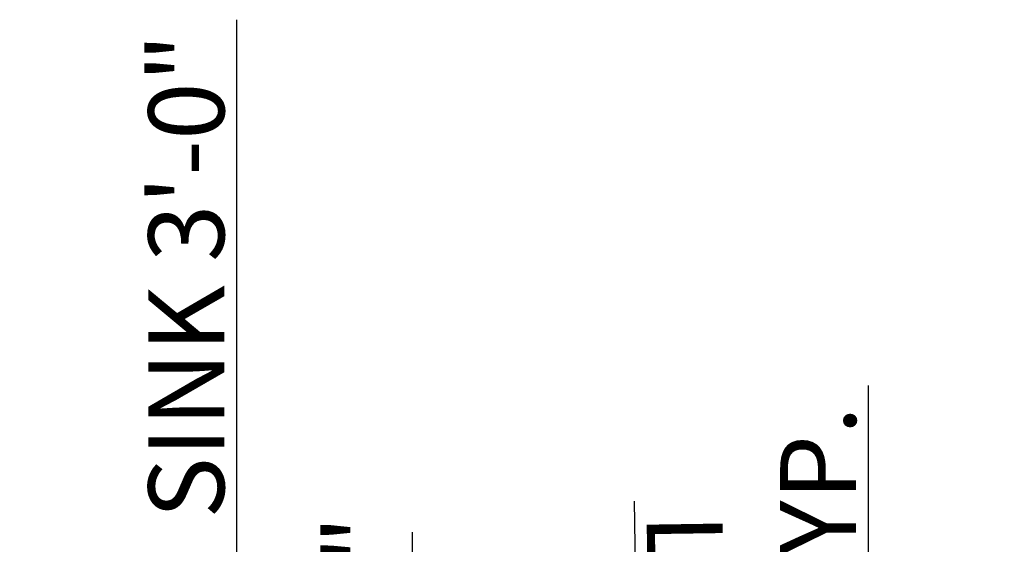
# Model space of a CAD drawing. Units: inches. Extents: x 2901 to 21549, y 2042 to 3828.
# Tile 9 of 10: x 3237 to 3704, y 3579 to 3828. Entities that reach past the tile are written whole.
import ezdxf

# ---------------------------------------------------------------- set-up
doc = ezdxf.new("R2010")
doc.units = ezdxf.units.IN
doc.layers.get('Defpoints').update_dxf_attribs({"color": 1})
doc.layers.add('A-ANNO-DIMS', color=2, linetype='Continuous', lineweight=18)
doc.styles.get("Standard").update_dxf_attribs({"font": 'arial.ttf'})
doc.dimstyles.new('ISO-25', dxfattribs={"dimtxt": 36, "dimasz": 5, "dimexe": 1.25, "dimexo": 0.625, "dimtad": 1, "dimdec": 0, "dimlunit": 3, "dimtxsty": 'Standard', "dimcen": 2.5, "dimadec": 0, "dimazin": 0, "dimtfac": 1, "dimtdec": 0, "dimtmove": 0, "dimatfit": 3, "dimfxl": 1, "dimarcsym": 0})

# ---------------------------------------------------------------- blocks, each defined once
blk = doc.blocks.new('*D36')
at = {"layer": 'A-ANNO-DIMS', "color": 0, "lineweight": -2, "transparency": 16777216}
for p, q in [((3639.47, 3192.64), (3639.47, 3654.44)), ((3634.69, 3192.64), (3640.72, 3192.64)), ((3639.47, 3161.64), (3639.47, 3187.64)), ((3634.69, 3156.64), (3640.72, 3156.64))]:
    blk.add_line(p, q, dxfattribs=at)
at = {"layer": 'A-ANNO-DIMS', "color": 0, "transparency": 16777216}
for points in [[(3638.64, 3187.64), (3640.3, 3187.64), (3639.47, 3192.64)], [(3638.64, 3161.64), (3640.3, 3161.64), (3639.47, 3156.64)]]:
    blk.add_solid(points, dxfattribs=at)
at = {"layer": 'Defpoints', "color": 0, "transparency": 16777216}
for p in [(3634.07, 3192.64), (3639.47, 3192.64), (3634.07, 3156.64)]:
    blk.add_point(p, dxfattribs=at)
at = {"layer": 'A-ANNO-DIMS', "color": 0, "transparency": 16777216, "insert": (3620.21, 3426.04), "char_height": 36, "attachment_point": 5, "rotation": 90}
blk.add_mtext('WINDOW 3\'-0" TYP.', dxfattribs=at)
blk = doc.blocks.new('*D42')
at = {"layer": 'A-ANNO-DIMS', "color": 0, "lineweight": -2, "transparency": 16777216}
for p, q in [((3533.42, 3266.44), (3528.38, 3599.53)), ((3535.49, 3266.47), (3532.17, 3266.42)), ((3533.62, 3253.49), (3533.5, 3261.44)), ((3535.76, 3248.52), (3532.44, 3248.47))]:
    blk.add_line(p, q, dxfattribs=at)
at = {"layer": 'A-ANNO-DIMS', "color": 0, "transparency": 16777216}
for points in [[(3534.33, 3261.45), (3532.66, 3261.43), (3533.42, 3266.44)], [(3534.45, 3253.5), (3532.78, 3253.48), (3533.69, 3248.49)]]:
    blk.add_solid(points, dxfattribs=at)
at = {"layer": 'Defpoints', "color": 0, "transparency": 16777216}
for p in [(3533.42, 3266.44), (3536.11, 3266.48), (3536.39, 3248.53)]:
    blk.add_point(p, dxfattribs=at)
at = {"layer": 'A-ANNO-DIMS', "color": 0, "transparency": 16777216, "insert": (3549.86, 3435.77), "char_height": 36, "attachment_point": 5, "rotation": 270.8679}
blk.add_mtext('LAV 1\'-6" TYP.', dxfattribs=at)
blk = doc.blocks.new('*D59')
at = {"layer": 'A-ANNO-DIMS', "color": 0, "lineweight": -2, "transparency": 16777216}
for p, q in [((3423.1, 3402.33), (3423.1, 3584.77)), ((3420.71, 3402.33), (3424.35, 3402.33)), ((3423.1, 3389.91), (3423.1, 3397.33)), ((3420.71, 3384.91), (3424.35, 3384.91))]:
    blk.add_line(p, q, dxfattribs=at)
at = {"layer": 'A-ANNO-DIMS', "color": 0, "transparency": 16777216}
for points in [[(3422.26, 3397.33), (3423.93, 3397.33), (3423.1, 3402.33)], [(3422.26, 3389.91), (3423.93, 3389.91), (3423.1, 3384.91)]]:
    blk.add_solid(points, dxfattribs=at)
at = {"layer": 'Defpoints', "color": 0, "transparency": 16777216}
for p in [(3420.08, 3402.33), (3423.1, 3402.33), (3420.08, 3384.91)]:
    blk.add_point(p, dxfattribs=at)
at = {"layer": 'A-ANNO-DIMS', "color": 0, "transparency": 16777216, "insert": (3403.86, 3496.05), "char_height": 36, "attachment_point": 5, "rotation": 90}
blk.add_mtext('1\'-5 1/2"', dxfattribs=at)
blk = doc.blocks.new('*D60')
at = {"layer": 'A-ANNO-DIMS', "color": 0, "lineweight": -2, "transparency": 16777216}
for p, q in [((3339.61, 3361.55), (3339.61, 3827.97)), ((3344.38, 3361.55), (3338.36, 3361.55)), ((3339.61, 3330.55), (3339.61, 3356.55)), ((3344.38, 3325.55), (3338.36, 3325.55))]:
    blk.add_line(p, q, dxfattribs=at)
at = {"layer": 'A-ANNO-DIMS', "color": 0, "transparency": 16777216}
for points in [[(3338.78, 3356.55), (3340.44, 3356.55), (3339.61, 3361.55)], [(3338.78, 3330.55), (3340.44, 3330.55), (3339.61, 3325.55)]]:
    blk.add_solid(points, dxfattribs=at)
at = {"layer": 'Defpoints', "color": 0, "transparency": 16777216}
for p in [(3339.61, 3361.55), (3345.01, 3361.55), (3345.01, 3325.55)]:
    blk.add_point(p, dxfattribs=at)
at = {"layer": 'A-ANNO-DIMS', "color": 0, "transparency": 16777216, "insert": (3320.36, 3597.26), "char_height": 36, "attachment_point": 5, "rotation": 90}
blk.add_mtext('KITCHEN SINK 3\'-0"', dxfattribs=at)

msp = doc.modelspace()

# ---------------------------------------------------------------- dimensions: what is measured, and where the dimension line sits
at = {"layer": 'A-ANNO-DIMS'}
for base, p1, p2, angle, text, picture, middle in [((3339.61, 3361.55), (3345.01, 3325.55), (3345.01, 3361.55), 90, 'KITCHEN SINK <>', '*D60', (3320.36, 3597.26)), ((3639.47, 3192.64), (3634.07, 3156.64), (3634.07, 3192.64), 90, 'WINDOW <> TYP.', '*D36', (3620.21, 3426.04)), ((3533.42, 3266.44), (3536.39, 3248.53), (3536.11, 3266.48), 90.8679, 'LAV <> TYP.', '*D42', (3549.86, 3435.77))]:
    dim = msp.add_linear_dim(base=base, p1=p1, p2=p2, angle=angle, text=text, dimstyle='ISO-25', override={"dimdec": 1, "dimlfac": 1, "dimrnd": 0, "dimzin": 1, "dimdsep": 46, "dimlunit": 4, "dimfrac": 2}, dxfattribs=at)
    dim.commit()
    dim.dimension.update_dxf_attribs({"geometry": picture, "text_midpoint": middle})
dim = msp.add_linear_dim(base=(3423.1, 3402.33), p1=(3420.08, 3384.91), p2=(3420.08, 3402.33), angle=90, dimstyle='ISO-25', override={"dimdec": 1, "dimlfac": 1, "dimrnd": 0, "dimzin": 1, "dimdsep": 46, "dimlunit": 4, "dimfrac": 2}, dxfattribs=at)
dim.commit()
dim.dimension.update_dxf_attribs({"geometry": '*D59', "text_midpoint": (3403.86, 3496.05)})

doc.saveas('drawing.dxf')
